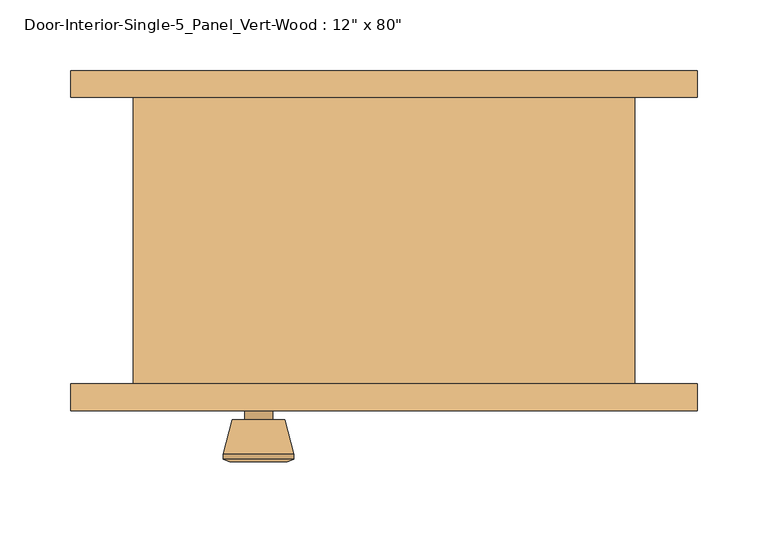
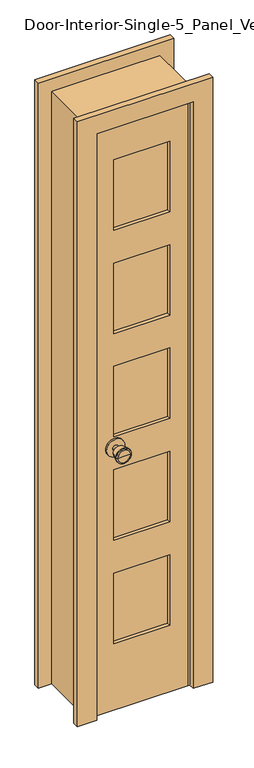
"""IFC4 building model written with IfcOpenShell, lengths in millimetres: door geometry."""

from ifc_helpers import new_model, si_unit, point, frame, frame_2d, origin, place, context, project, spatial, polyline, circle_curve, trimmed, segment, composite_curve, outline, extrude, faceted_brep, source, transform, mapped, element, save
from ifc_brep_helpers import plane_surface, cylinder_surface, revolved_surface, advanced_brep


def door_6ef897ee(model_context):
    return source(origin(), model_context, "Body", "SolidModel", [
        advanced_brep(
        [(-88.9, -57.5, 914.4), (-98.9, -57.5, 914.4), (-78.9, -57.5, 914.4), (-68.4241324, -8.5, 914.4), (-109.3758676, -8.5, 914.4), (-88.9, -8.5, 914.4), (-63.9, -10.3278681, 914.4), (-113.9, -10.3278681, 914.4), (-63.9, -13.7915463, 914.4), (-113.9, -13.7915463, 914.4), (-70.263764, -38.5, 914.4), (-107.536236, -38.5, 914.4), (-78.9, -38.5, 914.4), (-98.9, -38.5, 914.4)],
        [
            (0, 1),
            (1, 2, circle_curve(frame((-88.9, -57.5, 914.4), z_axis=(0.0, -1.0, 0.0), x_axis=(-1.0, 0.0, 0.0)), 10.0)),
            (2, 0),
            (2, 1, circle_curve(frame((-88.9, -57.5, 914.4), z_axis=(0.0, -1.0, 0.0), x_axis=(-1.0, 0.0, 0.0)), 10.0)),
            (3, 4, circle_curve(frame((-88.9, -8.5, 914.4), z_axis=(0.0, 1.0, 0.0), x_axis=(-1.0, 0.0, 0.0)), 20.4758676)),
            (4, 5),
            (5, 3),
            (4, 3, circle_curve(frame((-88.9, -8.5, 914.4), z_axis=(0.0, 1.0, 0.0), x_axis=(-1.0, 0.0, 0.0)), 20.4758676)),
            (6, 7, circle_curve(frame((-88.9, -10.3278681, 914.4), z_axis=(0.0, 1.0, 0.0), x_axis=(-1.0, 0.0, 0.0)), 25.0)),
            (7, 4),
            (3, 6),
            (7, 6, circle_curve(frame((-88.9, -10.3278681, 914.4), z_axis=(0.0, 1.0, 0.0), x_axis=(-1.0, 0.0, 0.0)), 25.0)),
            (8, 9, circle_curve(frame((-88.9, -13.7915463, 914.4), z_axis=(0.0, 1.0, 0.0), x_axis=(-1.0, 0.0, 0.0)), 25.0)),
            (9, 7),
            (6, 8),
            (9, 8, circle_curve(frame((-88.9, -13.7915463, 914.4), z_axis=(0.0, 1.0, 0.0), x_axis=(-1.0, 0.0, 0.0)), 25.0)),
            (10, 11, circle_curve(frame((-88.9, -38.5, 914.4), z_axis=(0.0, 1.0, 0.0), x_axis=(-1.0, 0.0, 0.0)), 18.636236)),
            (11, 9),
            (8, 10),
            (11, 10, circle_curve(frame((-88.9, -38.5, 914.4), z_axis=(0.0, 1.0, 0.0), x_axis=(-1.0, 0.0, 0.0)), 18.636236)),
            (12, 13, circle_curve(frame((-88.9, -38.5, 914.4), z_axis=(0.0, 1.0, 0.0), x_axis=(-1.0, 0.0, 0.0)), 10.0)),
            (13, 11),
            (10, 12),
            (13, 12, circle_curve(frame((-88.9, -38.5, 914.4), z_axis=(0.0, 1.0, 0.0), x_axis=(-1.0, 0.0, 0.0)), 10.0)),
            (1, 13),
            (12, 2),
        ],
        [
            plane_surface(frame((-88.9, -57.5, 914.4), z_axis=(0.0, -1.0, 0.0), x_axis=(-1.0, 0.0, 0.0))),
            plane_surface(frame((-88.9, -8.5, 914.4), z_axis=(0.0, 1.0, 0.0), x_axis=(-1.0, 0.0, 0.0))),
            revolved_surface(polyline([(-109.3758676, -8.5, 914.4), (-113.9, -10.3278681, 914.4)]), (-88.9, -57.5, 914.4), (0.0, -1.0, 0.0)),
            cylinder_surface(frame((-88.9, -57.5, 914.4), z_axis=(0.0, -1.0, 0.0), x_axis=(-1.0, 0.0, 0.0)), 25.0),
            revolved_surface(polyline([(-113.9, -13.7915463, 914.4), (-107.536236, -38.5, 914.4)]), (-88.9, -57.5, 914.4), (0.0, -1.0, 0.0)),
            plane_surface(frame((-88.9, -38.5, 914.4), z_axis=(0.0, -1.0, 0.0), x_axis=(-1.0, 0.0, 0.0))),
            cylinder_surface(frame((-88.9, -57.5, 914.4), z_axis=(0.0, -1.0, 0.0), x_axis=(-1.0, 0.0, 0.0)), 10.0),
        ],
        [
            (0, [[1, 2, 3]]),
            (0, [[-3, 4, -1]]),
            (1, [[5, 6, 7]]),
            (1, [[8, -7, -6]]),
            (2, [[9, 10, -5, 11]]),
            (2, [[12, -11, -8, -10]]),
            (3, [[13, 14, -9, 15]]),
            (3, [[16, -15, -12, -14]]),
            (4, [[17, 18, -13, 19]]),
            (4, [[20, -19, -16, -18]]),
            (5, [[21, 22, -17, 23]]),
            (5, [[24, -23, -20, -22]]),
            (6, [[-2, 25, -21, 26]]),
            (6, [[-4, -26, -24, -25]]),
        ],
    ),
        extrude(outline(composite_curve([segment(trimmed(circle_curve(frame_2d((914.4, -88.9)), 30.0), [point((914.4, -118.9))], [point((914.4, -58.9))], False, "CARTESIAN"), True, "CONTINUOUS"), segment(trimmed(circle_curve(frame_2d((914.4, -88.9)), 30.0), [point((914.4, -58.9))], [point((914.4, -118.9))], False, "CARTESIAN"), True, "CONTINUOUS")], self_intersect=False)), frame((0.0, -63.5, 0.0), z_axis=(0.0, 1.0, 0.0), x_axis=(0.0, 0.0, 1.0)), (0.0, 0.0, 1.0), 6.0),
        advanced_brep(
        [(-88.9, -104.425, 914.4), (-78.9, -104.425, 914.4), (-98.9, -104.425, 914.4), (-68.4241324, -153.425, 914.4), (-88.9, -153.425, 914.4), (-109.3758676, -153.425, 914.4), (-63.9, -151.5971319, 914.4), (-113.9, -151.5971319, 914.4), (-63.9, -148.1334537, 914.4), (-113.9, -148.1334537, 914.4), (-70.263764, -123.425, 914.4), (-107.536236, -123.425, 914.4), (-78.9, -123.425, 914.4), (-98.9, -123.425, 914.4)],
        [
            (0, 1),
            (1, 2, circle_curve(frame((-88.9, -104.425, 914.4), z_axis=(0.0, 1.0, 0.0), x_axis=(-1.0, 0.0, 0.0)), 10.0)),
            (2, 0),
            (2, 1, circle_curve(frame((-88.9, -104.425, 914.4), z_axis=(0.0, 1.0, 0.0), x_axis=(-1.0, 0.0, 0.0)), 10.0)),
            (3, 4),
            (4, 5),
            (5, 3, circle_curve(frame((-88.9, -153.425, 914.4), z_axis=(0.0, -1.0, 0.0), x_axis=(-1.0, 0.0, 0.0)), 20.4758676)),
            (3, 5, circle_curve(frame((-88.9, -153.425, 914.4), z_axis=(0.0, -1.0, 0.0), x_axis=(-1.0, 0.0, 0.0)), 20.4758676)),
            (6, 3),
            (5, 7),
            (7, 6, circle_curve(frame((-88.9, -151.5971319, 914.4), z_axis=(0.0, -1.0, 0.0), x_axis=(-1.0, 0.0, 0.0)), 25.0)),
            (6, 7, circle_curve(frame((-88.9, -151.5971319, 914.4), z_axis=(0.0, -1.0, 0.0), x_axis=(-1.0, 0.0, 0.0)), 25.0)),
            (8, 6),
            (7, 9),
            (9, 8, circle_curve(frame((-88.9, -148.1334537, 914.4), z_axis=(0.0, -1.0, 0.0), x_axis=(-1.0, 0.0, 0.0)), 25.0)),
            (8, 9, circle_curve(frame((-88.9, -148.1334537, 914.4), z_axis=(0.0, -1.0, 0.0), x_axis=(-1.0, 0.0, 0.0)), 25.0)),
            (10, 8),
            (9, 11),
            (11, 10, circle_curve(frame((-88.9, -123.425, 914.4), z_axis=(0.0, -1.0, 0.0), x_axis=(-1.0, 0.0, 0.0)), 18.636236)),
            (10, 11, circle_curve(frame((-88.9, -123.425, 914.4), z_axis=(0.0, -1.0, 0.0), x_axis=(-1.0, 0.0, 0.0)), 18.636236)),
            (12, 10),
            (11, 13),
            (13, 12, circle_curve(frame((-88.9, -123.425, 914.4), z_axis=(0.0, -1.0, 0.0), x_axis=(-1.0, 0.0, 0.0)), 10.0)),
            (12, 13, circle_curve(frame((-88.9, -123.425, 914.4), z_axis=(0.0, -1.0, 0.0), x_axis=(-1.0, 0.0, 0.0)), 10.0)),
            (1, 12),
            (13, 2),
        ],
        [
            plane_surface(frame((-88.9, -104.425, 914.4), z_axis=(0.0, 1.0, 0.0), x_axis=(-1.0, 0.0, 0.0))),
            plane_surface(frame((-88.9, -153.425, 914.4), z_axis=(0.0, -1.0, 0.0), x_axis=(-1.0, 0.0, 0.0))),
            revolved_surface(polyline([(-109.3758676, -153.425, 914.4), (-113.9, -151.5971319, 914.4)]), (-88.9, -104.425, 914.4), (0.0, 1.0, 0.0)),
            cylinder_surface(frame((-88.9, -104.425, 914.4), z_axis=(0.0, 1.0, 0.0), x_axis=(-1.0, 0.0, 0.0)), 25.0),
            revolved_surface(polyline([(-113.9, -148.1334537, 914.4), (-107.536236, -123.425, 914.4)]), (-88.9, -104.425, 914.4), (0.0, 1.0, 0.0)),
            plane_surface(frame((-88.9, -123.425, 914.4), z_axis=(0.0, 1.0, 0.0), x_axis=(-1.0, 0.0, 0.0))),
            cylinder_surface(frame((-88.9, -104.425, 914.4), z_axis=(0.0, 1.0, 0.0), x_axis=(-1.0, 0.0, 0.0)), 10.0),
        ],
        [
            (0, [[1, 2, 3]]),
            (0, [[-3, 4, -1]]),
            (1, [[5, 6, 7]]),
            (1, [[-6, -5, 8]]),
            (2, [[9, -7, 10, 11]]),
            (2, [[-10, -8, -9, 12]]),
            (3, [[13, -11, 14, 15]]),
            (3, [[-14, -12, -13, 16]]),
            (4, [[17, -15, 18, 19]]),
            (4, [[-18, -16, -17, 20]]),
            (5, [[21, -19, 22, 23]]),
            (5, [[-22, -20, -21, 24]]),
            (6, [[25, -23, 26, -2]]),
            (6, [[-26, -24, -25, -4]]),
        ],
    ),
        extrude(outline(composite_curve([segment(trimmed(circle_curve(frame_2d((914.4, -88.9)), 30.0), [point((914.4, -118.9))], [point((914.4, -58.9))], False, "CARTESIAN"), True, "CONTINUOUS"), segment(trimmed(circle_curve(frame_2d((914.4, -88.9)), 30.0), [point((914.4, -58.9))], [point((914.4, -118.9))], False, "CARTESIAN"), True, "CONTINUOUS")], self_intersect=False)), frame((0.0, -104.425, 0.0), z_axis=(0.0, 1.0, 0.0), x_axis=(0.0, 0.0, 1.0)), (0.0, 0.0, 1.0), 6.0),
        extrude(outline(polyline([(92.075, -75.1416667), (92.075, -86.7833333), (-92.075, -86.7833333), (-92.075, -75.1416667), (92.075, -75.1416667)])), frame((0.0, 0.0, 1668.145), z_axis=(0.0, 0.0, 1.0), x_axis=(1.0, 0.0, 0.0)), (0.0, 0.0, 1.0), 244.7925),
        extrude(outline(polyline([(92.075, -75.1416667), (92.075, -86.7833333), (-92.075, -86.7833333), (-92.075, -75.1416667), (92.075, -75.1416667)])), frame((0.0, 0.0, 1309.0525), z_axis=(0.0, 0.0, 1.0), x_axis=(1.0, 0.0, 0.0)), (0.0, 0.0, 1.0), 244.7925),
        extrude(outline(polyline([(92.075, -75.1416667), (92.075, -86.7833333), (-92.075, -86.7833333), (-92.075, -75.1416667), (92.075, -75.1416667)])), frame((0.0, 0.0, 590.8675), z_axis=(0.0, 0.0, 1.0), x_axis=(1.0, 0.0, 0.0)), (0.0, 0.0, 1.0), 244.7925),
        extrude(outline(polyline([(92.075, -75.1416667), (92.075, -86.7833333), (-92.075, -86.7833333), (-92.075, -75.1416667), (92.075, -75.1416667)])), frame((0.0, 0.0, 231.775), z_axis=(0.0, 0.0, 1.0), x_axis=(1.0, 0.0, 0.0)), (0.0, 0.0, 1.0), 244.7925),
        extrude(outline(polyline([(92.075, -75.1416667), (92.075, -86.7833333), (-92.075, -86.7833333), (-92.075, -75.1416667), (92.075, -75.1416667)])), frame((0.0, 0.0, 949.96), z_axis=(0.0, 0.0, 1.0), x_axis=(1.0, 0.0, 0.0)), (0.0, 0.0, 1.0), 244.7925),
        extrude(outline(polyline([(2032.0, -152.4), (0.0, -152.4), (0.0, 152.4), (2032.0, 152.4), (2032.0, -152.4)]), holes=[polyline([(1912.9375, -92.075), (1912.9375, 92.075), (1668.145, 92.075), (1668.145, -92.075), (1912.9375, -92.075)]), polyline([(476.5675, -92.075), (476.5675, 92.075), (231.775, 92.075), (231.775, -92.075), (476.5675, -92.075)]), polyline([(1194.7525, -92.075), (1194.7525, 92.075), (949.96, 92.075), (949.96, -92.075), (1194.7525, -92.075)]), polyline([(1553.845, -92.075), (1553.845, 92.075), (1309.0525, 92.075), (1309.0525, -92.075), (1553.845, -92.075)]), polyline([(835.66, -92.075), (835.66, 92.075), (590.8675, 92.075), (590.8675, -92.075), (835.66, -92.075)])]), frame((0.0, -98.425, 0.0), z_axis=(0.0, 1.0, 0.0), x_axis=(0.0, 0.0, 1.0)), (0.0, 0.0, 1.0), 34.925),
        faceted_brep([(177.8, -98.425, 0.0), (152.4, -98.425, 0.0), (152.4, -63.5, 0.0), (139.7, -63.5, 0.0), (139.7, -28.575, 0.0), (152.4, -28.575, 0.0), (152.4, 104.775, 0.0), (177.8, 104.775, 0.0), (177.8, 104.775, 2057.4), (177.8, -98.425, 2057.4), (152.4, 104.775, 2032.0), (-152.4, 104.775, 2032.0), (-152.4, 104.775, 0.0), (-177.8, 104.775, 0.0), (-177.8, 104.775, 2057.4), (152.4, -28.575, 2032.0), (139.7, -28.575, 2019.3), (-139.7, -28.575, 2019.3), (-139.7, -28.575, 0.0), (-152.4, -28.575, 0.0), (-152.4, -28.575, 2032.0), (139.7, -63.5, 2019.3), (152.4, -63.5, 2032.0), (-152.4, -63.5, 2032.0), (-152.4, -63.5, 0.0), (-139.7, -63.5, 0.0), (-139.7, -63.5, 2019.3), (152.4, -98.425, 2032.0), (-177.8, -98.425, 2057.4), (-177.8, -98.425, 0.0), (-152.4, -98.425, 0.0), (-152.4, -98.425, 2032.0)], [[[0, 1, 2, 3, 4, 5, 6, 7]], [[7, 8, 9, 0]], [[6, 10, 11, 12, 13, 14, 8, 7]], [[5, 15, 10, 6]], [[4, 16, 17, 18, 19, 20, 15, 5]], [[3, 21, 16, 4]], [[2, 22, 23, 24, 25, 26, 21, 3]], [[1, 27, 22, 2]], [[0, 9, 28, 29, 30, 31, 27, 1]], [[8, 14, 28, 9]], [[15, 20, 11, 10]], [[21, 26, 17, 16]], [[27, 31, 23, 22]], [[29, 13, 12, 19, 18, 25, 24, 30]], [[14, 13, 29, 28]], [[20, 19, 12, 11]], [[26, 25, 18, 17]], [[31, 30, 24, 23]]]),
        extrude(outline(polyline([(0.0, 222.25), (2101.85, 222.25), (2101.85, -222.25), (0.0, -222.25), (0.0, -158.75), (2038.35, -158.75), (2038.35, 158.75), (0.0, 158.75), (0.0, 222.25)])), frame((0.0, 104.775, 0.0), z_axis=(0.0, 1.0, 0.0), x_axis=(0.0, 0.0, 1.0)), (0.0, 0.0, 1.0), 19.05),
        extrude(outline(polyline([(0.0, 222.25), (2101.85, 222.25), (2101.85, -222.25), (0.0, -222.25), (0.0, -158.75), (2038.35, -158.75), (2038.35, 158.75), (0.0, 158.75), (0.0, 222.25)])), frame((0.0, -117.475, 0.0), z_axis=(0.0, 1.0, 0.0), x_axis=(0.0, 0.0, 1.0)), (0.0, 0.0, 1.0), 19.05),
    ])


if __name__ == "__main__":
    model = new_model("IFC4")
    model_context = context("Model", 3, world=origin())
    ifc_project = project(units=[si_unit("LENGTHUNIT", "METRE", prefix="MILLI")], contexts=[model_context])
    site = spatial("IfcSite", under=ifc_project)
    building = spatial("IfcBuilding", under=site)
    placement = place(None, origin())
    door_shape = door_6ef897ee(model_context)
    element("IfcDoor", 1, ObjectType="Door-Interior-Single-5_Panel_Vert-Wood : 12\" x 80\"", at=placement, inside=building, context=model_context, shape_type="MappedRepresentation", body=[
        mapped(door_shape, transform((0.0, 0.0, 0.0), x_axis=(1.0, 0.0, 0.0), y_axis=(0.0, 1.0, 0.0), z_axis=(0.0, 0.0, 1.0))),
    ])
    save(model, "model.ifc")

# Revit data of these elements
# Type "Door-Interior-Single-5_Panel_Vert-Wood : 12\" x 80\""
#   Type Mark = "8"
#   Assembly Code = "C1020300"
#   Analytic Construction = "Wooden"
#   Top Rail = 0' - 4 11/16"
#   Thickness = 0' - 1 3/8"
#   Thermal Resistance (R) = 2.5876 (h·ft²·°F)/BTU
#   Swing Angle [instance default] = 90.00°
#   Stiles = 0' - 2 3/8"
#   Rough Width = 1' - 2"
#   Rough Height = 6' - 9"
#   Intermediate Rail = 0' - 4 1/2"
#   Height = 6' - 8"
#   Width = 1' - 0"
#   Heat Transfer Coefficient (U) = 0.3865 BTU/(h·ft²·°F)
#   Bottom Rail = 0' - 9 1/8"
#   Trim Material = Cherry
#   Panel Material = Cherry
#   Frame Material = Cherry
#   Door Handle Material = Aluminum
#   Visual Light Transmittance = 0
#   Solar Heat Gain Coefficient = 0
#   Wall Closure = (empty or 0)
#   Function = (empty or 0)
# Element 1 (IfcDoor, "Door-Interior-Single-5_Panel_Vert-Wood : 12\" x 80\"")
#   Materials on its faces: "Cherry", "Aluminum"
# Materials
#   "Cherry": class "Wood", colour RGB 226 177 128, transparency 0, Description = "Prunus Serotina", Cost = 0
#   "Aluminum": class "Metal", colour RGB 247 247 247, transparency 0, Description = "Aluminum 6061", Cost = 0
